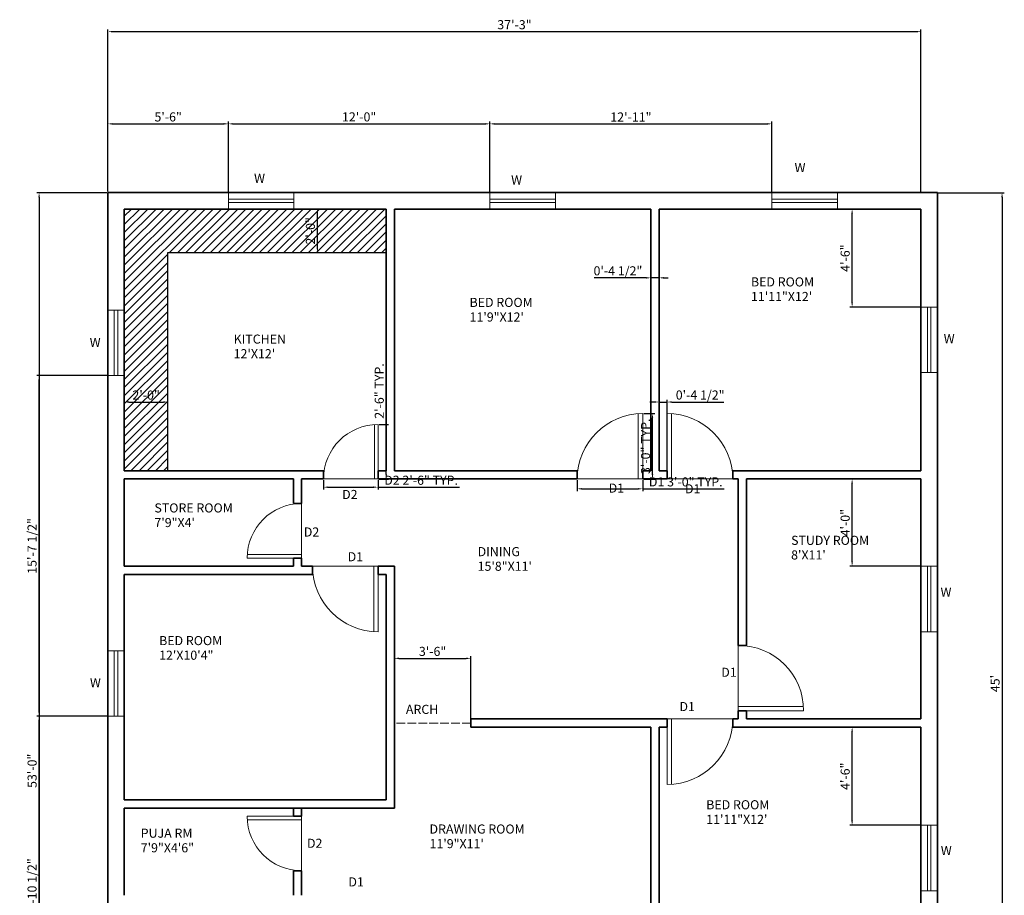
# Model space of a CAD drawing. Units: inches. Extents: x 2488 to 3029, y 1951 to 2721.
# Tile 2 of 2: x 2488 to 3029, y 2239 to 2721. Entities that reach past the tile are written whole.
import ezdxf

# ---------------------------------------------------------------- set-up
doc = ezdxf.new("R2010")
doc.units = ezdxf.units.IN
doc.header["$LTSCALE"] = 0.4
doc.linetypes.add('ACAD_ISO02W100', pattern=[15, 12, -3])
for name, color, linetype, lineweight in [('A-ANNO-DIMS', 52, 'Continuous', 18), ('A-ANNO-TEXT', 52, 'Continuous', 18), ('A-AREA-IDEN', 52, 'Continuous', 18), ('A-FLOR-FIXT', 8, 'Continuous', 25), ('A-FLOR-FIXT-PATT', 7, 'Continuous', 13), ('A-WALL-OVHD', 4, 'ACAD_ISO02W100', 18), ('doors', 4, 'Continuous', 18), ('wall', 5, 'Continuous', 35), ('windows', 8, 'Continuous', 18)]:
    doc.layers.add(name, color=color, linetype=linetype, lineweight=lineweight)
doc.styles.get("Standard").update_dxf_attribs({"font": 'arial.ttf', "height": 5})
doc.dimstyles.new('ISO-25', dxfattribs={"dimtxt": 5, "dimasz": 2.5, "dimexe": 1.25, "dimexo": 0.625, "dimtad": 1, "dimlunit": 3, "dimtxsty": 'Standard', "dimcen": 2.5, "dimadec": 0, "dimazin": 0, "dimtfac": 1, "dimtmove": 0, "dimatfit": 3, "dimfxl": 1, "dimarcsym": 0})

# ---------------------------------------------------------------- blocks, each defined once
blk = doc.blocks.new('*D6')
at = {"layer": 'A-ANNO-DIMS', "color": 0, "lineweight": -2, "transparency": 16777216}
for p, q in [((2993, 2625.69), (3029.19, 2625.69)), ((3027.94, 2623.19), (3027.94, 2088.19)), ((2993, 2085.69), (3029.19, 2085.69))]:
    blk.add_line(p, q, dxfattribs=at)
at = {"layer": 'A-ANNO-DIMS', "color": 0, "lineweight": 100, "transparency": 16777216}
for points in [[(3027.52, 2623.19), (3028.36, 2623.19), (3027.94, 2625.69)], [(3027.52, 2088.19), (3028.36, 2088.19), (3027.94, 2085.69)]]:
    blk.add_solid(points, dxfattribs=at)
at = {"layer": 'Defpoints', "color": 0, "lineweight": 100, "transparency": 16777216}
for p in [(2992.37, 2625.69), (2992.37, 2085.69), (3027.94, 2085.69)]:
    blk.add_point(p, dxfattribs=at)
at = {"layer": 'A-ANNO-DIMS', "color": 0, "transparency": 16777216, "insert": (3024.77, 2355.69), "char_height": 5, "attachment_point": 5, "rotation": 90}
blk.add_mtext("45'", dxfattribs=at)
blk = doc.blocks.new('*D7')
at = {"layer": 'A-ANNO-DIMS', "color": 0, "lineweight": -2, "transparency": 16777216}
for p, q in [((2536.37, 2626.32), (2536.37, 2715.51)), ((2538.87, 2714.26), (2980.87, 2714.26)), ((2983.37, 2626.32), (2983.37, 2715.51))]:
    blk.add_line(p, q, dxfattribs=at)
at = {"layer": 'A-ANNO-DIMS', "color": 0, "lineweight": 100, "transparency": 16777216}
for points in [[(2538.87, 2714.68), (2538.87, 2713.84), (2536.37, 2714.26)], [(2980.87, 2714.68), (2980.87, 2713.84), (2983.37, 2714.26)]]:
    blk.add_solid(points, dxfattribs=at)
at = {"layer": 'Defpoints', "color": 0, "lineweight": 100, "transparency": 16777216}
for p in [(2983.37, 2714.26), (2536.37, 2625.69), (2983.37, 2625.69)]:
    blk.add_point(p, dxfattribs=at)
at = {"layer": 'A-ANNO-DIMS', "color": 0, "transparency": 16777216, "insert": (2759.87, 2717.44), "char_height": 5, "attachment_point": 5}
blk.add_mtext('37\'-3"', dxfattribs=at)
blk = doc.blocks.new('WIN-36IN-9IN-WALL')
for p, q in [((0, 36), (0, 0)), ((9, 36), (0, 36)), ((3.5, 36), (3.5, 0)), ((5.5, 36), (5.5, 0)), ((9, 0), (9, 36)), ((0, 0), (9, 0))]:
    blk.add_line(p, q)
blk = doc.blocks.new('DOOR-SWING-30IN')
for p, q in [((28, 29.93), (28, 0)), ((30, 30), (30, 0)), ((30, 0), (0, 0))]:
    blk.add_line(p, q)
blk.add_arc((30, 0), 30, 90, 180)
blk = doc.blocks.new('DOOR-SWING-36IN')
for p, q in [((33.6, 35.92), (33.6, 0)), ((36, 36), (36, 0)), ((36, 0), (0, 0))]:
    blk.add_line(p, q)
blk.add_arc((36, 0), 36, 90, 180)
blk = doc.blocks.new('*D13')
at = {"layer": 'A-ANNO-DIMS', "color": 0, "lineweight": -2, "transparency": 16777216}
for p, q in [((2794.37, 2467.57), (2794.37, 2461.54)), ((2830.37, 2467.57), (2830.37, 2461.54)), ((2796.87, 2462.79), (2827.87, 2462.79)), ((2830.37, 2462.79), (2875.22, 2462.79))]:
    blk.add_line(p, q, dxfattribs=at)
at = {"layer": 'A-ANNO-DIMS', "color": 0, "lineweight": 100, "transparency": 16777216}
for points in [[(2796.87, 2463.21), (2796.87, 2462.38), (2794.37, 2462.79)], [(2827.87, 2463.21), (2827.87, 2462.38), (2830.37, 2462.79)]]:
    blk.add_solid(points, dxfattribs=at)
at = {"layer": 'Defpoints', "color": 0, "lineweight": 100, "transparency": 16777216}
for p in [(2794.37, 2468.19), (2830.37, 2468.19), (2830.37, 2462.79)]:
    blk.add_point(p, dxfattribs=at)
at = {"layer": 'A-ANNO-DIMS', "color": 0, "transparency": 16777216, "insert": (2854.05, 2465.97), "char_height": 5, "attachment_point": 5}
blk.add_mtext('D1 3\'-0" TYP.', dxfattribs=at)
blk = doc.blocks.new('*D14')
at = {"layer": 'A-ANNO-DIMS', "color": 0, "lineweight": -2, "transparency": 16777216}
for p, q in [((2831, 2504.19), (2837.02, 2504.19)), ((2835.77, 2470.69), (2835.77, 2501.69)), ((2831, 2468.19), (2837.02, 2468.19))]:
    blk.add_line(p, q, dxfattribs=at)
at = {"layer": 'A-ANNO-DIMS', "color": 0, "lineweight": 100, "transparency": 16777216}
for points in [[(2835.36, 2501.69), (2836.19, 2501.69), (2835.77, 2504.19)], [(2835.36, 2470.69), (2836.19, 2470.69), (2835.77, 2468.19)]]:
    blk.add_solid(points, dxfattribs=at)
at = {"layer": 'Defpoints', "color": 0, "lineweight": 100, "transparency": 16777216}
for p in [(2830.37, 2504.19), (2835.77, 2504.19), (2830.37, 2468.19)]:
    blk.add_point(p, dxfattribs=at)
at = {"layer": 'A-ANNO-DIMS', "color": 0, "transparency": 16777216, "insert": (2832.59, 2486.19), "char_height": 5, "attachment_point": 5, "rotation": 90}
blk.add_mtext('3\'-0" TYP.', dxfattribs=at)
blk = doc.blocks.new('*D15')
at = {"layer": 'A-ANNO-DIMS', "color": 0, "lineweight": -2, "transparency": 16777216}
for p, q in [((2654.87, 2467.57), (2654.87, 2462.44)), ((2657.37, 2463.69), (2682.37, 2463.69)), ((2684.87, 2467.57), (2684.87, 2462.44)), ((2684.87, 2463.69), (2729.72, 2463.69))]:
    blk.add_line(p, q, dxfattribs=at)
at = {"layer": 'A-ANNO-DIMS', "color": 0, "lineweight": 100, "transparency": 16777216}
for points in [[(2657.37, 2464.11), (2657.37, 2463.28), (2654.87, 2463.69)], [(2682.37, 2464.11), (2682.37, 2463.28), (2684.87, 2463.69)]]:
    blk.add_solid(points, dxfattribs=at)
at = {"layer": 'Defpoints', "color": 0, "lineweight": 100, "transparency": 16777216}
for p in [(2654.87, 2468.19), (2684.87, 2468.19), (2684.87, 2463.69)]:
    blk.add_point(p, dxfattribs=at)
at = {"layer": 'A-ANNO-DIMS', "color": 0, "transparency": 16777216, "insert": (2708.55, 2466.87), "char_height": 5, "attachment_point": 5}
blk.add_mtext('D2 2\'-6" TYP.', dxfattribs=at)
blk = doc.blocks.new('*D16')
at = {"layer": 'A-ANNO-DIMS', "color": 0, "lineweight": -2, "transparency": 16777216}
for p, q in [((2689.37, 2498.19), (2689.37, 2532.51)), ((2685.5, 2498.19), (2690.62, 2498.19)), ((2689.37, 2470.69), (2689.37, 2495.69)), ((2685.5, 2468.19), (2690.62, 2468.19))]:
    blk.add_line(p, q, dxfattribs=at)
at = {"layer": 'A-ANNO-DIMS', "color": 0, "lineweight": 100, "transparency": 16777216}
for points in [[(2688.96, 2495.69), (2689.79, 2495.69), (2689.37, 2498.19)], [(2688.96, 2470.69), (2689.79, 2470.69), (2689.37, 2468.19)]]:
    blk.add_solid(points, dxfattribs=at)
at = {"layer": 'Defpoints', "color": 0, "lineweight": 100, "transparency": 16777216}
for p in [(2684.87, 2498.19), (2689.37, 2498.19), (2684.87, 2468.19)]:
    blk.add_point(p, dxfattribs=at)
at = {"layer": 'A-ANNO-DIMS', "color": 0, "transparency": 16777216, "insert": (2686.2, 2516.6), "char_height": 5, "attachment_point": 5, "rotation": 90}
blk.add_mtext('2\'-6" TYP.', dxfattribs=at)
blk = doc.blocks.new('*D17')
at = {"layer": 'A-ANNO-DIMS', "color": 0, "lineweight": -2, "transparency": 16777216}
for p, q in [((2536.37, 2626.32), (2536.37, 2664.79)), ((2538.87, 2663.54), (2600.08, 2663.54)), ((2602.58, 2626.32), (2602.58, 2664.79))]:
    blk.add_line(p, q, dxfattribs=at)
at = {"layer": 'A-ANNO-DIMS', "color": 0, "lineweight": 100, "transparency": 16777216}
for points in [[(2538.87, 2663.96), (2538.87, 2663.13), (2536.37, 2663.54)], [(2600.08, 2663.96), (2600.08, 2663.13), (2602.58, 2663.54)]]:
    blk.add_solid(points, dxfattribs=at)
at = {"layer": 'Defpoints', "color": 0, "lineweight": 100, "transparency": 16777216}
for p in [(2602.58, 2663.54), (2536.37, 2625.69), (2602.58, 2625.69)]:
    blk.add_point(p, dxfattribs=at)
at = {"layer": 'A-ANNO-DIMS', "color": 0, "transparency": 16777216, "insert": (2569.48, 2666.72), "char_height": 5, "attachment_point": 5}
blk.add_mtext('5\'-6"', dxfattribs=at)
blk = doc.blocks.new('*D18')
at = {"layer": 'A-ANNO-DIMS', "color": 0, "lineweight": -2, "transparency": 16777216}
for p, q in [((2602.58, 2626.32), (2602.58, 2664.79)), ((2605.08, 2663.54), (2743.87, 2663.54)), ((2746.37, 2626.32), (2746.37, 2664.79))]:
    blk.add_line(p, q, dxfattribs=at)
at = {"layer": 'A-ANNO-DIMS', "color": 0, "lineweight": 100, "transparency": 16777216}
for points in [[(2605.08, 2663.96), (2605.08, 2663.13), (2602.58, 2663.54)], [(2743.87, 2663.96), (2743.87, 2663.13), (2746.37, 2663.54)]]:
    blk.add_solid(points, dxfattribs=at)
at = {"layer": 'Defpoints', "color": 0, "lineweight": 100, "transparency": 16777216}
for p in [(2746.37, 2663.54), (2602.58, 2625.69), (2746.37, 2625.69)]:
    blk.add_point(p, dxfattribs=at)
at = {"layer": 'A-ANNO-DIMS', "color": 0, "transparency": 16777216, "insert": (2674.48, 2666.72), "char_height": 5, "attachment_point": 5}
blk.add_mtext('12\'-0"', dxfattribs=at)
blk = doc.blocks.new('*D19')
at = {"layer": 'A-ANNO-DIMS', "color": 0, "lineweight": -2, "transparency": 16777216}
for p, q in [((2746.37, 2626.32), (2746.37, 2664.79)), ((2748.87, 2663.54), (2898.92, 2663.54)), ((2901.42, 2626.32), (2901.42, 2664.79))]:
    blk.add_line(p, q, dxfattribs=at)
at = {"layer": 'A-ANNO-DIMS', "color": 0, "lineweight": 100, "transparency": 16777216}
for points in [[(2748.87, 2663.96), (2748.87, 2663.13), (2746.37, 2663.54)], [(2898.92, 2663.96), (2898.92, 2663.13), (2901.42, 2663.54)]]:
    blk.add_solid(points, dxfattribs=at)
at = {"layer": 'Defpoints', "color": 0, "lineweight": 100, "transparency": 16777216}
for p in [(2901.42, 2663.54), (2746.37, 2625.69), (2901.42, 2625.69)]:
    blk.add_point(p, dxfattribs=at)
at = {"layer": 'A-ANNO-DIMS', "color": 0, "transparency": 16777216, "insert": (2823.9, 2666.68), "char_height": 5, "attachment_point": 5}
blk.add_mtext('12\'-11"', dxfattribs=at)
blk = doc.blocks.new('*D21')
at = {"layer": 'A-ANNO-DIMS', "color": 0, "lineweight": -2, "transparency": 16777216}
for p, q in [((2535.75, 2337.69), (2497.27, 2337.69)), ((2498.52, 2149.53), (2498.52, 2335.19)), ((2535.75, 2147.03), (2497.27, 2147.03))]:
    blk.add_line(p, q, dxfattribs=at)
at = {"layer": 'A-ANNO-DIMS', "color": 0, "lineweight": 100, "transparency": 16777216}
for points in [[(2498.11, 2335.19), (2498.94, 2335.19), (2498.52, 2337.69)], [(2498.11, 2149.53), (2498.94, 2149.53), (2498.52, 2147.03)]]:
    blk.add_solid(points, dxfattribs=at)
at = {"layer": 'Defpoints', "color": 0, "lineweight": 100, "transparency": 16777216}
for p in [(2498.52, 2337.69), (2536.37, 2337.69), (2536.37, 2147.03)]:
    blk.add_point(p, dxfattribs=at)
at = {"layer": 'A-ANNO-DIMS', "color": 0, "transparency": 16777216, "insert": (2495.31, 2242.36), "char_height": 5, "attachment_point": 5, "rotation": 90}
blk.add_mtext('15\'-10 1/2"', dxfattribs=at)
blk = doc.blocks.new('*D22')
at = {"layer": 'A-ANNO-DIMS', "color": 0, "lineweight": -2, "transparency": 16777216}
for p, q in [((2535.75, 2525.06), (2497.27, 2525.06)), ((2498.52, 2340.19), (2498.52, 2522.56)), ((2535.75, 2337.69), (2497.27, 2337.69))]:
    blk.add_line(p, q, dxfattribs=at)
at = {"layer": 'A-ANNO-DIMS', "color": 0, "lineweight": 100, "transparency": 16777216}
for points in [[(2498.11, 2522.56), (2498.94, 2522.56), (2498.52, 2525.06)], [(2498.11, 2340.19), (2498.94, 2340.19), (2498.52, 2337.69)]]:
    blk.add_solid(points, dxfattribs=at)
at = {"layer": 'Defpoints', "color": 0, "lineweight": 100, "transparency": 16777216}
for p in [(2498.52, 2525.06), (2536.37, 2525.06), (2536.37, 2337.69)]:
    blk.add_point(p, dxfattribs=at)
at = {"layer": 'A-ANNO-DIMS', "color": 0, "transparency": 16777216, "insert": (2495.31, 2431.38), "char_height": 5, "attachment_point": 5, "rotation": 90}
blk.add_mtext('15\'-7 1/2"', dxfattribs=at)
blk = doc.blocks.new('*D23')
at = {"layer": 'A-ANNO-DIMS', "color": 0, "lineweight": -2, "transparency": 16777216}
for p, q in [((2982.75, 2616.69), (2944.27, 2616.69)), ((2945.52, 2565.19), (2945.52, 2614.19)), ((2982.75, 2562.69), (2944.27, 2562.69))]:
    blk.add_line(p, q, dxfattribs=at)
at = {"layer": 'A-ANNO-DIMS', "color": 0, "lineweight": 100, "transparency": 16777216}
for points in [[(2945.11, 2614.19), (2945.94, 2614.19), (2945.52, 2616.69)], [(2945.11, 2565.19), (2945.94, 2565.19), (2945.52, 2562.69)]]:
    blk.add_solid(points, dxfattribs=at)
at = {"layer": 'Defpoints', "color": 0, "lineweight": 100, "transparency": 16777216}
for p in [(2945.52, 2616.69), (2983.37, 2616.69), (2983.37, 2562.69)]:
    blk.add_point(p, dxfattribs=at)
at = {"layer": 'A-ANNO-DIMS', "color": 0, "transparency": 16777216, "insert": (2942.35, 2589.69), "char_height": 5, "attachment_point": 5, "rotation": 90}
blk.add_mtext('4\'-6"', dxfattribs=at)
blk = doc.blocks.new('*D24')
at = {"layer": 'A-ANNO-DIMS', "color": 0, "lineweight": -2, "transparency": 16777216}
for p, q in [((2982.75, 2468.19), (2944.27, 2468.19)), ((2945.52, 2422.69), (2945.52, 2465.69)), ((2982.75, 2420.19), (2944.27, 2420.19))]:
    blk.add_line(p, q, dxfattribs=at)
at = {"layer": 'A-ANNO-DIMS', "color": 0, "lineweight": 100, "transparency": 16777216}
for points in [[(2945.11, 2465.69), (2945.94, 2465.69), (2945.52, 2468.19)], [(2945.11, 2422.69), (2945.94, 2422.69), (2945.52, 2420.19)]]:
    blk.add_solid(points, dxfattribs=at)
at = {"layer": 'Defpoints', "color": 0, "lineweight": 100, "transparency": 16777216}
for p in [(2945.52, 2468.19), (2983.37, 2468.19), (2983.37, 2420.19)]:
    blk.add_point(p, dxfattribs=at)
at = {"layer": 'A-ANNO-DIMS', "color": 0, "transparency": 16777216, "insert": (2942.35, 2444.19), "char_height": 5, "attachment_point": 5, "rotation": 90}
blk.add_mtext('4\'-0"', dxfattribs=at)
blk = doc.blocks.new('*D25')
at = {"layer": 'A-ANNO-DIMS', "color": 0, "lineweight": -2, "transparency": 16777216}
for p, q in [((2982.75, 2331.69), (2944.27, 2331.69)), ((2945.52, 2280.19), (2945.52, 2329.19)), ((2982.75, 2277.69), (2944.27, 2277.69))]:
    blk.add_line(p, q, dxfattribs=at)
at = {"layer": 'A-ANNO-DIMS', "color": 0, "lineweight": 100, "transparency": 16777216}
for points in [[(2945.11, 2329.19), (2945.94, 2329.19), (2945.52, 2331.69)], [(2945.11, 2280.19), (2945.94, 2280.19), (2945.52, 2277.69)]]:
    blk.add_solid(points, dxfattribs=at)
at = {"layer": 'Defpoints', "color": 0, "lineweight": 100, "transparency": 16777216}
for p in [(2945.52, 2331.69), (2983.37, 2331.69), (2983.37, 2277.69)]:
    blk.add_point(p, dxfattribs=at)
at = {"layer": 'A-ANNO-DIMS', "color": 0, "transparency": 16777216, "insert": (2942.35, 2304.69), "char_height": 5, "attachment_point": 5, "rotation": 90}
blk.add_mtext('4\'-6"', dxfattribs=at)
blk = doc.blocks.new('*D31')
at = {"layer": 'A-ANNO-DIMS', "color": 0, "lineweight": -2, "transparency": 16777216}
for p, q in [((2535.75, 2625.69), (2497.27, 2625.69)), ((2498.52, 2623.19), (2498.52, 1992.19)), ((2693.25, 1989.69), (2497.27, 1989.69))]:
    blk.add_line(p, q, dxfattribs=at)
at = {"layer": 'A-ANNO-DIMS', "color": 0, "lineweight": 100, "transparency": 16777216}
for points in [[(2498.11, 2623.19), (2498.94, 2623.19), (2498.52, 2625.69)], [(2498.11, 1992.19), (2498.94, 1992.19), (2498.52, 1989.69)]]:
    blk.add_solid(points, dxfattribs=at)
at = {"layer": 'Defpoints', "color": 0, "lineweight": 100, "transparency": 16777216}
for p in [(2536.37, 2625.69), (2498.52, 1989.69), (2693.87, 1989.69)]:
    blk.add_point(p, dxfattribs=at)
at = {"layer": 'A-ANNO-DIMS', "color": 0, "transparency": 16777216, "insert": (2495.34, 2307.69), "char_height": 5, "attachment_point": 5, "rotation": 90}
blk.add_mtext('53\'-0"', dxfattribs=at)
blk = doc.blocks.new('*D32')
at = {"layer": 'A-ANNO-DIMS', "color": 0, "lineweight": -2, "transparency": 16777216}
for p, q in [((2545.37, 2473.32), (2545.37, 2511.79)), ((2569.37, 2473.32), (2569.37, 2511.79)), ((2547.87, 2510.54), (2566.87, 2510.54))]:
    blk.add_line(p, q, dxfattribs=at)
at = {"layer": 'A-ANNO-DIMS', "color": 0, "lineweight": 100, "transparency": 16777216}
for points in [[(2547.87, 2510.96), (2547.87, 2510.13), (2545.37, 2510.54)], [(2566.87, 2510.96), (2566.87, 2510.13), (2569.37, 2510.54)]]:
    blk.add_solid(points, dxfattribs=at)
at = {"layer": 'Defpoints', "color": 0, "lineweight": 100, "transparency": 16777216}
for p in [(2569.37, 2510.54), (2545.37, 2472.69), (2569.37, 2472.69)]:
    blk.add_point(p, dxfattribs=at)
at = {"layer": 'A-ANNO-DIMS', "color": 0, "transparency": 16777216, "insert": (2557.37, 2513.72), "char_height": 5, "attachment_point": 5}
blk.add_mtext('2\'-0"', dxfattribs=at)
blk = doc.blocks.new('*D33')
at = {"layer": 'A-ANNO-DIMS', "color": 0, "lineweight": -2, "transparency": 16777216}
for p, q in [((2688.75, 2616.69), (2650.27, 2616.69)), ((2651.52, 2595.19), (2651.52, 2614.19)), ((2688.75, 2592.69), (2650.27, 2592.69))]:
    blk.add_line(p, q, dxfattribs=at)
at = {"layer": 'A-ANNO-DIMS', "color": 0, "lineweight": 100, "transparency": 16777216}
for points in [[(2651.11, 2614.19), (2651.94, 2614.19), (2651.52, 2616.69)], [(2651.11, 2595.19), (2651.94, 2595.19), (2651.52, 2592.69)]]:
    blk.add_solid(points, dxfattribs=at)
at = {"layer": 'Defpoints', "color": 0, "lineweight": 100, "transparency": 16777216}
for p in [(2651.52, 2616.69), (2689.37, 2616.69), (2689.37, 2592.69)]:
    blk.add_point(p, dxfattribs=at)
at = {"layer": 'A-ANNO-DIMS', "color": 0, "transparency": 16777216, "insert": (2648.35, 2604.69), "char_height": 5, "attachment_point": 5, "rotation": 90}
blk.add_mtext('2\'-0"', dxfattribs=at)
blk = doc.blocks.new('*D34')
at = {"layer": 'A-ANNO-DIMS', "color": 0, "lineweight": -2, "transparency": 16777216}
for p, q in [((2693.87, 2332.32), (2693.87, 2370.79)), ((2696.37, 2369.54), (2733.37, 2369.54)), ((2735.87, 2332.32), (2735.87, 2370.79))]:
    blk.add_line(p, q, dxfattribs=at)
at = {"layer": 'A-ANNO-DIMS', "color": 0, "lineweight": 100, "transparency": 16777216}
for points in [[(2696.37, 2369.96), (2696.37, 2369.13), (2693.87, 2369.54)], [(2733.37, 2369.96), (2733.37, 2369.13), (2735.87, 2369.54)]]:
    blk.add_solid(points, dxfattribs=at)
at = {"layer": 'Defpoints', "color": 0, "lineweight": 100, "transparency": 16777216}
for p in [(2735.87, 2369.54), (2693.87, 2331.69), (2735.87, 2331.69)]:
    blk.add_point(p, dxfattribs=at)
at = {"layer": 'A-ANNO-DIMS', "color": 0, "transparency": 16777216, "insert": (2714.87, 2372.72), "char_height": 5, "attachment_point": 5}
blk.add_mtext('3\'-6"', dxfattribs=at)
blk = doc.blocks.new('*D35')
at = {"layer": 'A-ANNO-DIMS', "color": 0, "lineweight": -2, "transparency": 16777216}
for p, q in [((2834.87, 2616.07), (2834.87, 2577.59)), ((2839.37, 2616.07), (2839.37, 2577.59)), ((2832.37, 2578.84), (2803.68, 2578.84)), ((2839.37, 2578.84), (2834.87, 2578.84)), ((2841.87, 2578.84), (2844.37, 2578.84))]:
    blk.add_line(p, q, dxfattribs=at)
at = {"layer": 'A-ANNO-DIMS', "color": 0, "lineweight": 100, "transparency": 16777216}
for points in [[(2832.37, 2579.26), (2832.37, 2578.43), (2834.87, 2578.84)], [(2841.87, 2579.26), (2841.87, 2578.43), (2839.37, 2578.84)]]:
    blk.add_solid(points, dxfattribs=at)
at = {"layer": 'Defpoints', "color": 0, "lineweight": 100, "transparency": 16777216}
for p in [(2834.87, 2616.69), (2839.37, 2616.69), (2834.87, 2578.84)]:
    blk.add_point(p, dxfattribs=at)
at = {"layer": 'A-ANNO-DIMS', "color": 0, "transparency": 16777216, "insert": (2816.78, 2582.05), "char_height": 5, "attachment_point": 5}
blk.add_mtext('0\'-4 1/2"', dxfattribs=at)
blk = doc.blocks.new('*D41')
at = {"layer": 'A-ANNO-DIMS', "color": 0, "lineweight": -2, "transparency": 16777216}
for p, q in [((2839.37, 2473.32), (2839.37, 2511.79)), ((2843.87, 2473.32), (2843.87, 2511.79)), ((2836.87, 2510.54), (2834.37, 2510.54)), ((2839.37, 2510.54), (2843.87, 2510.54)), ((2846.37, 2510.54), (2875.07, 2510.54))]:
    blk.add_line(p, q, dxfattribs=at)
at = {"layer": 'A-ANNO-DIMS', "color": 0, "lineweight": 100, "transparency": 16777216}
for points in [[(2836.87, 2510.96), (2836.87, 2510.13), (2839.37, 2510.54)], [(2846.37, 2510.96), (2846.37, 2510.13), (2843.87, 2510.54)]]:
    blk.add_solid(points, dxfattribs=at)
at = {"layer": 'Defpoints', "color": 0, "lineweight": 100, "transparency": 16777216}
for p in [(2843.87, 2510.54), (2839.37, 2472.69), (2843.87, 2472.69)]:
    blk.add_point(p, dxfattribs=at)
at = {"layer": 'A-ANNO-DIMS', "color": 0, "transparency": 16777216, "insert": (2861.97, 2513.75), "char_height": 5, "attachment_point": 5}
blk.add_mtext('0\'-4 1/2"', dxfattribs=at)

msp = doc.modelspace()

# ---------------------------------------------------------------- hatches: boundary and pattern name
at = {"layer": 'A-FLOR-FIXT-PATT'}
h = msp.add_hatch(dxfattribs=at)
h.set_pattern_fill('ANSI31', color=256)
h.paths.add_polyline_path([(2689.374, 2616.694), (2545.374, 2616.694), (2545.374, 2472.694), (2569.374, 2472.694), (2569.374, 2592.694), (2689.374, 2592.694)])

# ---------------------------------------------------------------- linework, layer by layer
at = {"layer": 'A-FLOR-FIXT'}
for p, q in [((2569.374, 2592.694), (2689.374, 2592.694)), ((2569.374, 2472.694), (2569.374, 2592.694))]:
    msp.add_line(p, q, dxfattribs=at)
at = {"layer": 'A-WALL-OVHD'}
msp.add_line((2735.874, 2333.944), (2693.874, 2333.944), dxfattribs=at)
at = {"layer": 'wall'}
for p, q in [((2536.374, 2625.694), (2992.374, 2625.694)), ((2536.374, 2085.694), (2536.374, 2625.694)), ((2992.374, 2625.694), (2992.374, 2085.694)), ((2545.374, 2616.694), (2689.374, 2616.694)), ((2545.374, 2472.694), (2545.374, 2616.694)), ((2689.374, 2472.694), (2689.374, 2616.694)), ((2689.374, 2472.694), (2689.374, 2616.694)), ((2689.374, 2472.694), (2689.374, 2616.694)), ((2693.874, 2472.694), (2693.874, 2616.694)), ((2693.874, 2472.694), (2693.874, 2616.694)), ((2693.874, 2616.694), (2834.874, 2616.694)), ((2834.874, 2472.694), (2834.874, 2616.694)), ((2839.374, 2472.694), (2839.374, 2616.694)), ((2839.374, 2616.694), (2983.374, 2616.694)), ((2983.374, 2616.694), (2983.374, 2472.694)), ((2545.374, 2472.694), (2654.874, 2472.694)), ((2654.874, 2472.694), (2654.874, 2468.194)), ((2684.874, 2472.694), (2684.874, 2468.194)), ((2684.874, 2472.694), (2689.374, 2472.694)), ((2693.874, 2472.694), (2794.374, 2472.694)), ((2794.374, 2472.694), (2794.374, 2468.194)), ((2830.374, 2472.694), (2830.374, 2468.194)), ((2830.374, 2472.694), (2834.874, 2472.694)), ((2839.374, 2472.694), (2843.874, 2472.694)), ((2843.874, 2472.694), (2843.874, 2468.194)), ((2879.874, 2472.694), (2879.874, 2468.194)), ((2879.874, 2472.694), (2983.374, 2472.694)), ((2545.374, 2468.194), (2638.374, 2468.194)), ((2545.374, 2420.194), (2545.374, 2468.194)), ((2638.374, 2454.694), (2638.374, 2468.194)), ((2638.374, 2454.694), (2638.374, 2468.194)), ((2642.874, 2468.194), (2654.874, 2468.194)), ((2642.874, 2454.694), (2642.874, 2468.194)), ((2642.874, 2454.694), (2642.874, 2468.194)), ((2684.874, 2468.194), (2794.374, 2468.194)), ((2830.374, 2468.194), (2843.874, 2468.194)), ((2879.874, 2468.194), (2882.874, 2468.194)), ((2882.874, 2468.194), (2882.874, 2376.694)), ((2887.374, 2468.194), (2887.374, 2376.694)), ((2887.374, 2468.194), (2983.374, 2468.194)), ((2983.374, 2468.194), (2983.374, 2336.194)), ((2638.374, 2454.694), (2642.874, 2454.694)), ((2545.374, 2420.194), (2638.374, 2420.194)), ((2638.374, 2420.194), (2638.374, 2424.694)), ((2638.374, 2420.194), (2638.374, 2424.694)), ((2638.374, 2424.694), (2642.874, 2424.694)), ((2642.874, 2420.194), (2642.874, 2424.694)), ((2642.874, 2420.194), (2642.874, 2424.694)), ((2642.874, 2420.194), (2648.874, 2420.194)), ((2648.874, 2415.694), (2648.874, 2420.194)), ((2684.874, 2415.694), (2684.874, 2420.194)), ((2684.874, 2420.194), (2693.874, 2420.194)), ((2693.874, 2336.194), (2693.874, 2420.194)), ((2545.374, 2415.694), (2648.874, 2415.694)), ((2545.374, 2291.694), (2545.374, 2415.694)), ((2684.874, 2415.694), (2689.374, 2415.694)), ((2689.374, 2291.694), (2689.374, 2415.694)), ((2689.374, 2291.694), (2689.374, 2415.694)), ((2882.874, 2376.694), (2887.374, 2376.694)), ((2882.874, 2340.694), (2887.374, 2340.694)), ((2882.874, 2340.694), (2882.874, 2336.194)), ((2887.374, 2340.694), (2887.374, 2336.194)), ((2693.874, 2336.194), (2693.874, 2331.694)), ((2735.874, 2336.194), (2843.874, 2336.194)), ((2735.874, 2336.194), (2735.874, 2331.694)), ((2843.874, 2331.694), (2843.874, 2336.194)), ((2879.874, 2331.694), (2879.874, 2336.194)), ((2879.874, 2336.194), (2882.874, 2336.194)), ((2887.374, 2336.194), (2983.374, 2336.194)), ((2693.874, 2287.194), (2693.874, 2331.694)), ((2735.874, 2331.694), (2834.874, 2331.694)), ((2834.874, 2187.694), (2834.874, 2331.694)), ((2839.374, 2187.694), (2839.374, 2331.694)), ((2839.374, 2331.694), (2843.874, 2331.694)), ((2879.874, 2331.694), (2983.374, 2331.694)), ((2983.374, 2331.694), (2983.374, 2187.694)), ((2545.374, 2291.694), (2689.374, 2291.694)), ((2545.374, 2287.194), (2638.374, 2287.194)), ((2545.374, 2239.194), (2545.374, 2287.194)), ((2642.874, 2287.194), (2638.374, 2287.194)), ((2638.374, 2282.694), (2638.374, 2287.194)), ((2642.874, 2287.194), (2693.874, 2287.194)), ((2642.874, 2282.694), (2642.874, 2287.194)), ((2642.874, 2282.694), (2638.374, 2282.694)), ((2638.374, 2239.194), (2638.374, 2252.694)), ((2642.874, 2252.694), (2638.374, 2252.694)), ((2642.874, 2239.194), (2642.874, 2252.694))]:
    msp.add_line(p, q, dxfattribs=at)

# ---------------------------------------------------------------- block references
at = {"layer": 'doors'}
for name, p in [('DOOR-SWING-36IN', (2794.374, 2468.194)), ('DOOR-SWING-30IN', (2654.874, 2468.194))]:
    msp.add_blockref(name, p, dxfattribs=at)
at = {"layer": 'doors', "extrusion": (0, 0, -1), "zscale": -1}
msp.add_blockref('DOOR-SWING-36IN', (-2879.874, 2468.194), dxfattribs=at)
for name, p, rotation in [('DOOR-SWING-30IN', (-2642.874, 2454.694), 269.9999999999992), ('DOOR-SWING-36IN', (-2648.874, 2420.194), 180)]:
    msp.add_blockref(name, p, dxfattribs=dict(at, rotation=rotation))
at = {"layer": 'doors'}
for name, p, rotation in [('DOOR-SWING-36IN', (2882.874, 2376.694), 269.9999999999936), ('DOOR-SWING-36IN', (2879.874, 2336.194), 180), ('DOOR-SWING-30IN', (2642.874, 2252.694), 89.99999999999903)]:
    msp.add_blockref(name, p, dxfattribs=dict(at, rotation=rotation))
at = {"layer": 'windows'}
for p, rotation in [((2602.584, 2625.694), 270.0000000000021), ((2746.374, 2625.694), 270.0000000000031), ((2901.422, 2625.694), 270.0000000000003), ((2545.374, 2561.064), 180), ((2992.374, 2420.194), 180), ((2545.374, 2373.694), 180), ((2992.374, 2277.694), 180)]:
    msp.add_blockref('WIN-36IN-9IN-WALL', p, dxfattribs=dict(at, rotation=rotation))
msp.add_blockref('WIN-36IN-9IN-WALL', (2983.374, 2526.694), dxfattribs=at)

# ---------------------------------------------------------------- texts
at = {"layer": 'A-ANNO-TEXT'}
for s, p in [('W', (2913.886, 2636.973)), ('W', (2616.725, 2631.056)), ('W', (2758.066, 2630.157)), ('W', (2526.351, 2540.822)), ('W', (2995.877, 2542.886)), ('D1', (2811.683, 2460.692)), ('D1', (2853.646, 2460.311)), ('D2', (2665.131, 2457.168)), ('D2', (2644.085, 2436.537)), ('D1', (2668.173, 2422.926)), ('W', (2994.138, 2403.463)), ('D1', (2873.569, 2359.376)), ('W', (2526.487, 2353.632)), ('ARCH', (2700.194, 2338.98)), ('D1', (2850.608, 2340.518)), ('D2', (2645.812, 2265.315)), ('W', (2994.286, 2261.291)), ('D1', (2668.584, 2244.066))]:
    msp.add_text(s, height=5, dxfattribs=at).set_placement(p)
at = {"layer": 'A-AREA-IDEN'}
for s, p in [('BED ROOM', (2889.908, 2574.111)), ('11\'11"X12\'', (2889.908, 2566.079)), ('BED ROOM', (2735.198, 2562.844)), ('11\'9"X12\'', (2735.198, 2554.812)), ('KITCHEN', (2605.49, 2542.659)), ("12'X12'", (2605.49, 2534.627)), ('STORE ROOM', (2561.931, 2449.776)), ('7\'9"X4\'', (2561.931, 2441.744)), ('STUDY ROOM', (2911.975, 2431.952)), ('DINING ', (2739.631, 2425.735)), ("8'X11'", (2911.975, 2423.92)), ('15\'8"X11\'', (2739.631, 2417.703)), ('BED ROOM', (2564.513, 2376.797)), ('12\'X10\'4"', (2564.513, 2368.765)), ('BED ROOM', (2865.314, 2286.512)), ('11\'11"X12\'', (2865.314, 2278.48)), ('PUJA RM', (2554.407, 2270.871)), ('DRAWING ROOM', (2713.188, 2273.155)), ('11\'9"X11\'', (2713.188, 2265.123)), ('7\'9"X4\'6"', (2554.407, 2262.839))]:
    msp.add_text(s, height=5, dxfattribs=at).set_placement(p)

# ---------------------------------------------------------------- dimensions: what is measured, and where the dimension line sits
at = {"layer": 'A-ANNO-DIMS'}
for base, p1, p2, override, picture, middle in [((2983.374, 2714.259), (2536.374, 2625.694), (2983.374, 2625.694), {"dimclrd": 0, "dimclre": 0, "dimclrt": 0}, '*D7', (2759.874, 2717.438)), ((2602.584, 2663.544), (2536.374, 2625.694), (2602.584, 2625.694), {"dimdec": 1, "dimlfac": 1, "dimrnd": 0, "dimzin": 1, "dimdsep": 46, "dimlunit": 4, "dimfrac": 2}, '*D17', (2569.479, 2666.722)), ((2746.374, 2663.544), (2602.584, 2625.694), (2746.374, 2625.694), {"dimdec": 1, "dimlfac": 1, "dimrnd": 0, "dimzin": 1, "dimdsep": 46, "dimlunit": 4, "dimfrac": 2}, '*D18', (2674.479, 2666.722)), ((2901.422, 2663.544), (2746.374, 2625.694), (2901.422, 2625.694), {"dimdec": 1, "dimlfac": 1, "dimrnd": 0, "dimzin": 1, "dimdsep": 46, "dimlunit": 4, "dimfrac": 2}, '*D19', (2823.898, 2666.679)), ((2843.874, 2510.544), (2839.374, 2472.694), (2843.874, 2472.694), {"dimdec": 1, "dimlfac": 1, "dimrnd": 0, "dimzin": 1, "dimdsep": 46, "dimlunit": 4, "dimfrac": 2}, '*D41', (2861.97, 2513.754)), ((2569.374, 2510.544), (2545.374, 2472.694), (2569.374, 2472.694), {"dimdec": 1, "dimlfac": 1, "dimrnd": 0, "dimzin": 1, "dimdsep": 46, "dimlunit": 4, "dimfrac": 2}, '*D32', (2557.374, 2513.722)), ((2735.874, 2369.544), (2693.874, 2331.694), (2735.874, 2331.694), {"dimdec": 1, "dimlfac": 1, "dimrnd": 0, "dimzin": 1, "dimdsep": 46, "dimlunit": 4, "dimfrac": 2}, '*D34', (2714.874, 2372.723))]:
    dim = msp.add_linear_dim(base=base, p1=p1, p2=p2, dimstyle='ISO-25', override=override, dxfattribs=at)
    dim.commit()
    dim.dimension.update_dxf_attribs({"geometry": picture, "text_midpoint": middle})
for base, p1, p2, angle, override, picture, middle in [((2498.524, 1989.694), (2536.374, 2625.694), (2693.874, 1989.694), 90, {"dimdec": 1, "dimlfac": 1, "dimrnd": 0, "dimzin": 1, "dimdsep": 46, "dimlunit": 4, "dimfrac": 2}, '*D31', (2495.344, 2307.694)), ((3027.941, 2085.694), (2992.374, 2625.694), (2992.374, 2085.694), 90, {"dimclrd": 0, "dimclre": 0, "dimclrt": 0}, '*D6', (3024.773, 2355.694)), ((2651.524, 2616.694), (2689.374, 2592.694), (2689.374, 2616.694), 90, {"dimdec": 1, "dimlfac": 1, "dimrnd": 0, "dimzin": 1, "dimdsep": 46, "dimlunit": 4, "dimfrac": 2}, '*D33', (2648.346, 2604.694)), ((2834.874, 2578.844), (2839.374, 2616.694), (2834.874, 2616.694), 180, {"dimdec": 1, "dimlfac": 1, "dimrnd": 0, "dimzin": 1, "dimdsep": 46, "dimlunit": 4, "dimfrac": 2}, '*D35', (2816.777, 2582.054)), ((2945.524, 2616.694), (2983.374, 2562.694), (2983.374, 2616.694), 90, {"dimdec": 1, "dimlfac": 1, "dimrnd": 0, "dimzin": 1, "dimdsep": 46, "dimlunit": 4, "dimfrac": 2}, '*D23', (2942.346, 2589.694)), ((2498.524, 2525.064), (2536.374, 2337.694), (2536.374, 2525.064), 90, {"dimdec": 1, "dimlfac": 1, "dimrnd": 0, "dimzin": 1, "dimdsep": 46, "dimlunit": 4, "dimfrac": 2}, '*D22', (2495.313, 2431.379)), ((2945.524, 2468.194), (2983.374, 2420.194), (2983.374, 2468.194), 90, {"dimdec": 1, "dimlfac": 1, "dimrnd": 0, "dimzin": 1, "dimdsep": 46, "dimlunit": 4, "dimfrac": 2}, '*D24', (2942.346, 2444.194)), ((2498.524, 2337.694), (2536.374, 2147.028), (2536.374, 2337.694), 90, {"dimdec": 1, "dimlfac": 1, "dimrnd": 0, "dimzin": 1, "dimdsep": 46, "dimlunit": 4, "dimfrac": 2}, '*D21', (2495.313, 2242.361)), ((2945.524, 2331.694), (2983.374, 2277.694), (2983.374, 2331.694), 90, {"dimdec": 1, "dimlfac": 1, "dimrnd": 0, "dimzin": 1, "dimdsep": 46, "dimlunit": 4, "dimfrac": 2}, '*D25', (2942.346, 2304.694))]:
    dim = msp.add_linear_dim(base=base, p1=p1, p2=p2, angle=angle, dimstyle='ISO-25', override=override, dxfattribs=at)
    dim.commit()
    dim.dimension.update_dxf_attribs({"geometry": picture, "text_midpoint": middle})
for base, p1, p2, picture, middle in [((2689.374, 2498.194), (2684.874, 2468.194), (2684.874, 2498.194), '*D16', (2686.196, 2516.6)), ((2835.774, 2504.194), (2830.374, 2468.194), (2830.374, 2504.194), '*D14', (2832.594, 2486.194))]:
    dim = msp.add_linear_dim(base=base, p1=p1, p2=p2, angle=90, text='<> TYP.', dimstyle='ISO-25', override={"dimdec": 1, "dimlfac": 1, "dimrnd": 0, "dimzin": 1, "dimdsep": 46, "dimlunit": 4, "dimfrac": 2}, dxfattribs=at)
    dim.commit()
    dim.dimension.update_dxf_attribs({"geometry": picture, "text_midpoint": middle})
for base, p1, p2, text, picture, middle in [((2684.874, 2463.694), (2654.874, 2468.194), (2684.874, 2468.194), 'D2 <> TYP.', '*D15', (2708.548, 2466.872)), ((2830.374, 2462.794), (2794.374, 2468.194), (2830.374, 2468.194), 'D1 <> TYP.', '*D13', (2854.048, 2465.973))]:
    dim = msp.add_linear_dim(base=base, p1=p1, p2=p2, text=text, dimstyle='ISO-25', override={"dimdec": 1, "dimlfac": 1, "dimrnd": 0, "dimzin": 1, "dimdsep": 46, "dimlunit": 4, "dimfrac": 2}, dxfattribs=at)
    dim.commit()
    dim.dimension.update_dxf_attribs({"geometry": picture, "text_midpoint": middle})

doc.saveas('drawing.dxf')
